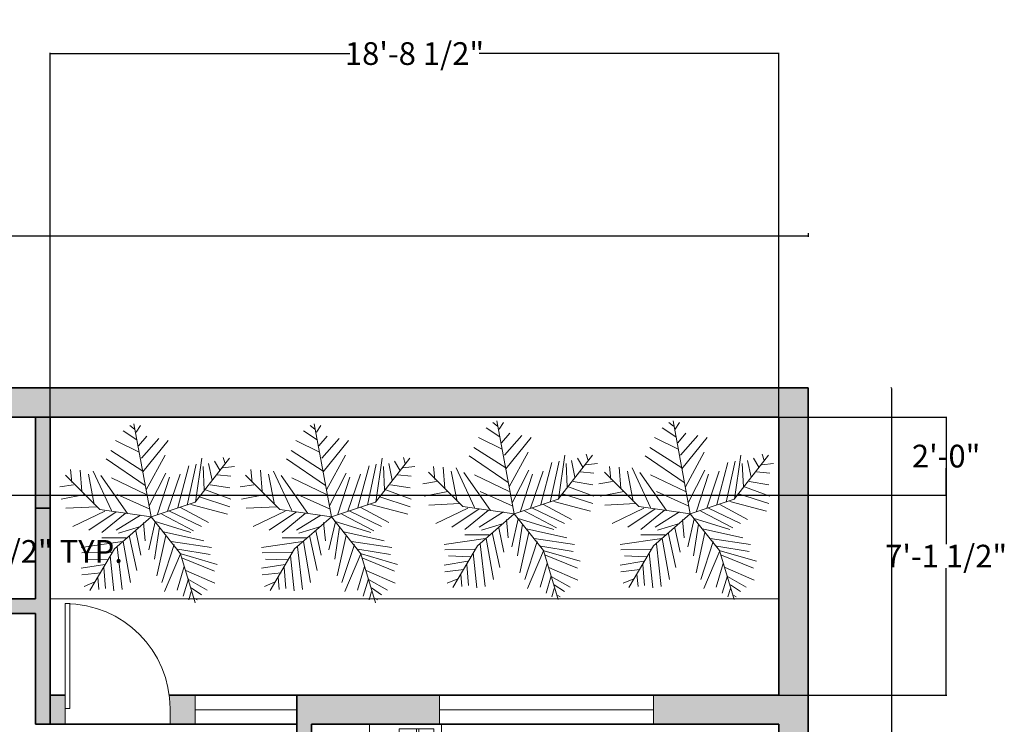
# Model space of a CAD drawing. Units: inches. Extents: x 1319 to 2030, y 219 to 1069.
# Tile 28 of 28: x 1727 to 2030, y 852 to 1069. Entities that reach past the tile are written whole.
import ezdxf

# ---------------------------------------------------------------- set-up
doc = ezdxf.new("R2010")
doc.units = ezdxf.units.IN
doc.header["$MEASUREMENT"] = 0
doc.layers.get('0').update_dxf_attribs({"color": 12})
for name, color, linetype, lineweight in [('A-ANNO-DIMS', 2, 'Continuous', 18), ('A-GLAZ', 4, 'Continuous', 18), ('A-WALL-PATT', 252, 'Continuous', 13), ('C-PROP', 7, 'Continuous', 35), ('doors', 252, 'Continuous', 18), ('furniture', 250, 'Continuous', 18), ('lawn', 82, 'Continuous', 13), ('walls', 250, 'Continuous', 35)]:
    doc.layers.add(name, color=color, linetype=linetype, lineweight=lineweight)
doc.styles.get("Standard").update_dxf_attribs({"font": 'arial.ttf'})
doc.dimstyles.get("Standard").update_dxf_attribs({"dimtxt": 7, "dimasz": 0.18, "dimexe": 0.18, "dimexo": 0.0625, "dimgap": 0.09, "dimtad": 0, "dimtih": 1, "dimtoh": 1, "dimzin": 0, "dimdsep": 46, "dimlunit": 3, "dimtxsty": 'Standard', "dimcen": 0.09, "dimadec": 0, "dimazin": 0, "dimtfac": 1, "dimtofl": 0, "dimtmove": 0, "dimatfit": 3, "dimfxl": 1, "dimtolj": 1, "dimtzin": 0, "dimarcsym": 0})

# ---------------------------------------------------------------- blocks, each defined once
blk = doc.blocks.new('*U2')
for p, q in [((0, 0), (0, -6)), ((40, 0), (40, -6))]:
    blk.add_line(p, q)
blk.add_lwpolyline([(0, 0), (0, 40), (1.75, 40), (1.75, 0)], close=True)
blk.add_arc((0, 0), 40, 0, 90)
blk = doc.blocks.new('*U27')
for p, q in [((-10.186, 53.64), (-13.084, 55.962)), ((0, 0), (-10.5, 57)), ((-9.099, 51.782), (-6.563, 55.962)), ((-8.737, 47.138), (-17.069, 52.711)), ((-7.65, 43.423), (-2.578, 49.46)), ((-7.288, 39.707), (-21.778, 46.673)), ((-5.839, 35.992), (4.667, 48.067)), ((-5.114, 27.632), (10.463, 46.673)), ((-5.114, 28.097), (-24.676, 40.636)), ((-2.941, 16.486), (8.652, 37.85)), ((44.153, 36.456), (45.239, 32.741)), ((-3.665, 19.273), (-27.574, 35.527)), ((16.259, 5.805), (23.142, 31.348)), ((22.055, 7.198), (27.489, 32.277)), ((27, 9), (48, 36)), ((27.127, 9.056), (31.112, 35.992)), ((31.836, 30.883), (32.561, 16.486)), ((35.096, 32.741), (37.27, 22.524)), ((38.719, 34.134), (41.979, 28.561)), ((43.791, 29.954), (51.036, 30.883)), ((-31.5, 4.5), (-52.5, 25.5)), ((-48.585, 21.131), (-49.309, 29.026)), ((-43.513, 28.561), (-42.427, 15.558)), ((-38.442, 26.239), (-34.819, 7.663)), ((-35.544, 28.097), (-24.314, 3.947)), ((-14.533, 2.09), (-30.834, 25.31)), ((-1.129, 6.734), (9.014, 26.704)), ((3.942, 1.625), (11.187, 24.381)), ((10.101, 3.483), (17.708, 26.239)), ((40.53, 25.775), (48.862, 24.846)), ((-47.498, 19.737), (-55.83, 18.344)), ((-24.314, 23.917), (-2.941, 13.7)), ((36.183, 19.737), (48.137, 17.88)), ((-40.615, 13.7), (-55.105, 10.913)), ((-20.691, 13.7), (-1.129, 4.876)), ((29.662, 12.307), (48.137, 6.269)), ((33.285, 16.486), (48.862, 10.913)), ((-33.37, 6.269), (-52.207, 5.34)), ((0, 0), (27, 9)), ((24.229, 7.663), (46.688, 1.625)), ((-28.299, 3.483), (-47.86, -5.805)), ((-21.416, 3.018), (-38.079, -8.128)), ((0, 0), (-31.5, 4.5)), ((-15.982, 2.09), (-30.11, -9.521)), ((0, 0), (-22.5, -19.5)), ((-6.563, 1.161), (-21.416, -8.128)), ((0, 0), (18, -22.5)), ((6.478, 1.625), (26.04, -8.592)), ((11.187, 3.483), (30.749, -5.805)), ((18.07, 5.805), (35.096, -3.483)), ((-6.563, -5.805), (-19.967, -9.985)), ((-4.752, -3.483), (-3.665, -14.629)), ((2.493, -3.019), (-1.491, -20.202)), ((1.769, -2.555), (24.229, -9.521)), ((-13.446, -11.378), (-8.737, -32.741)), ((-9.461, -8.592), (-6.201, -23.453)), ((5.029, -6.27), (2.131, -25.775)), ((9.014, -11.378), (3.58, -35.992)), ((7.565, -9.056), (32.198, -14.629)), ((-17.431, -15.094), (-42.789, -18.809)), ((-15.257, -12.772), (-30.11, -12.772)), ((-17.069, -15.094), (-12.721, -40.172)), ((14.085, -16.951), (6.478, -40.172)), ((12.274, -15.094), (36.907, -18.809)), ((-24.314, -21.596), (-42.427, -22.06)), ((-22.5, -19.5), (-37.5, -45)), ((-25.038, -23.918), (-22.865, -45.281)), ((-20.691, -18.345), (-17.793, -44.352)), ((18.07, -22.524), (8.289, -45.745)), ((16.259, -19.738), (36.183, -22.989)), ((18, -22.5), (27, -52.5)), ((18.433, -22.524), (40.53, -29.026)), ((-28.299, -29.026), (-42.789, -31.348)), ((-26.849, -26.24), (-40.253, -25.775)), ((19.157, -25.311), (38.719, -33.206)), ((-30.834, -34.135), (-42.427, -35.528)), ((-29.023, -30.884), (-27.936, -43.887)), ((20.244, -30.419), (15.897, -44.816)), ((21.331, -32.741), (39.081, -40.636)), ((-34.457, -39.708), (-40.978, -42.494)), ((-32.646, -36.921), (-31.921, -44.352)), ((22.78, -37.85), (19.519, -48.532)), ((22.78, -38.314), (34.372, -44.816)), ((24.591, -45.745), (23.142, -50.854)), ((24.591, -43.423), (30.749, -47.603)), ((26.764, -49.925), (28.213, -50.854))]:
    blk.add_line(p, q)
blk = doc.blocks.new('*D28')
at = {"layer": 'A-ANNO-DIMS', "color": 0, "lineweight": -2, "transparency": 16777216}
for p, q in [((1369.84, 1002.94), (1369.84, 1001.77)), ((1370.02, 1001.95), (1663.81, 1001.95)), ((1969.66, 1001.95), (1675.87, 1001.95)), ((1969.84, 1002.94), (1969.84, 1001.77))]:
    blk.add_line(p, q, dxfattribs=at)
at = {"layer": 'A-ANNO-DIMS', "color": 0, "transparency": 16777216}
for points in [[(1370.02, 1001.98), (1370.02, 1001.92), (1369.84, 1001.95)], [(1969.66, 1001.98), (1969.66, 1001.92), (1969.84, 1001.95)]]:
    blk.add_solid(points, dxfattribs=at)
at = {"layer": 'Defpoints', "color": 0, "transparency": 16777216}
for p in [(1369.84, 1003), (1969.84, 1003), (1969.84, 1001.95)]:
    blk.add_point(p, dxfattribs=at)
at = {"layer": 'A-ANNO-DIMS', "color": 0, "transparency": 16777216, "insert": (1669.84, 1001.95), "char_height": 7, "attachment_point": 5}
blk.add_mtext("\\A1;50'", dxfattribs=at)
blk = doc.blocks.new('*D29')
at = {"layer": 'A-ANNO-DIMS', "color": 0, "lineweight": -2, "transparency": 16777216}
for p, q in [((1995.58, 955.23), (1995.33, 955.23)), ((1995.51, 955.05), (1995.51, 628.88)), ((1995.51, 295.41), (1995.51, 621.58)), ((1995.58, 295.23), (1995.33, 295.23))]:
    blk.add_line(p, q, dxfattribs=at)
at = {"layer": 'A-ANNO-DIMS', "color": 0, "transparency": 16777216}
for points in [[(1995.48, 955.05), (1995.54, 955.05), (1995.51, 955.23)], [(1995.48, 295.41), (1995.54, 295.41), (1995.51, 295.23)]]:
    blk.add_solid(points, dxfattribs=at)
at = {"layer": 'Defpoints', "color": 0, "transparency": 16777216}
for p in [(1995.64, 955.23), (1995.51, 295.23), (1995.64, 295.23)]:
    blk.add_point(p, dxfattribs=at)
at = {"layer": 'A-ANNO-DIMS', "color": 0, "transparency": 16777216, "insert": (1995.51, 625.23), "char_height": 7, "attachment_point": 5}
blk.add_mtext("\\A1;55'", dxfattribs=at)
blk = doc.blocks.new('PLASMA-LARGE')
at = {"layer": 'furniture'}
for p, q in [((-7.26, 0), (7.26, 0)), ((-21, -2.5), (21, -2.5)), ((-21, -2.5), (-21, -3.5)), ((-21, -3.5), (21, -3.5)), ((-18.61, -1), (18.61, -1)), ((-8, -1), (-8, -0.74)), ((-8, -3.5), (-8, -4.76)), ((-7.26, -5.5), (7.26, -5.5)), ((8, -1), (8, -0.74)), ((8, -3.5), (8, -4.76)), ((21, -2.5), (21, -3.5))]:
    blk.add_line(p, q, dxfattribs=at)
for centre, radius, start, end in [((-7.26, -0.74), 0.744, 90, 180), ((7.26, -0.74), 0.744, 0, 90), ((-13.97, -11.05), 11.07, 114.76019, 129.41749), ((-7.26, -4.76), 0.744, 180, 270), ((7.26, -4.76), 0.744, 270, 0), ((13.97, -11.05), 11.07, 50.58251, 65.23981)]:
    blk.add_arc(centre, radius, start, end, dxfattribs=at)
blk = doc.blocks.new('STUDY-STATION')
h = blk.add_hatch(color=256)
h.dxf.hatch_style = 1
h.paths.add_polyline_path([(29.65, 37, 0.288578), (17.34, 37)])
h = blk.add_hatch(color=256)
h.dxf.hatch_style = 1
h.paths.add_polyline_path([(33.33, 21.74), (24.73, 21.74), (24.73, 18.77), (33.33, 18.77)])
for p, q in [((13.58, 39.93), (0, 39.93)), ((13.58, 17.73), (13.58, 39.93)), ((20.6, 38.07), (17.92, 42.38)), ((17.92, 42.38), (21.92, 38.58)), ((27.56, 41.97), (24.23, 38.82)), ((25.39, 38.48), (27.56, 41.97)), ((13.58, 37.53), (1.44, 37.53)), ((1.44, 37.53), (1.44, 26.9)), ((17.34, 37), (17.34, 25.83)), ((26.82, 37.82), (20.17, 37.82)), ((29.65, 25.83), (29.65, 37)), ((13.58, 32.99), (1.44, 32.99)), ((1.44, 32.99), (1.44, 32.21)), ((1.44, 32.21), (13.58, 32.21)), ((13.58, 26.9), (13.58, 32.99)), ((17.34, 32.49), (15.81, 32.49)), ((15.81, 32.49), (15.81, 31.73)), ((15.81, 31.73), (17.34, 31.73)), ((17.34, 32.49), (17.34, 32.49)), ((29.65, 32.49), (31.18, 32.49)), ((31.18, 31.73), (29.65, 31.73)), ((31.18, 32.49), (31.18, 31.73)), ((1.44, 26.9), (13.58, 26.9)), ((17.34, 25.83), (29.65, 25.83)), ((14.64, 17.73), (14.64, 22.88)), ((14.64, 22.88), (34.27, 22.88)), ((24.73, 17.73), (24.73, 21.74)), ((24.73, 21.74), (33.33, 21.74)), ((33.33, 21.74), (33.33, 17.73)), ((34.27, 22.88), (34.27, 17.73)), ((24.73, 18.77), (33.33, 18.77)), ((0, 17.73), (36.53, 17.73)), ((36.53, 17.73), (36.53, 0))]:
    blk.add_line(p, q)
for centre, radius, start, end in [((23.49, 27.23), 11.55, 57.806, 122.194), ((23.49, 25.83), 0.688, 180, 0)]:
    blk.add_arc(centre, radius, start, end)
at = {"xscale": -0.3577737849257557, "yscale": 0.3577737849257557, "zscale": 0.3577737849257557, "rotation": 180}
blk.add_blockref('PLASMA-LARGE', (19.61, 8.15), dxfattribs=at)
blk = doc.blocks.new('*D40')
at = {"layer": 'A-ANNO-DIMS', "color": 0, "lineweight": -2, "transparency": 16777216}
for p, q in [((1703.84, 919.51), (1708.35, 919.51)), ((1708.17, 919.33), (1708.17, 908.58)), ((1708.17, 890.41), (1708.17, 901.15)), ((1703.84, 890.23), (1708.35, 890.23))]:
    blk.add_line(p, q, dxfattribs=at)
at = {"layer": 'A-ANNO-DIMS', "color": 0, "transparency": 16777216}
for points in [[(1708.14, 919.33), (1708.2, 919.33), (1708.17, 919.51)], [(1708.14, 890.41), (1708.2, 890.41), (1708.17, 890.23)]]:
    blk.add_solid(points, dxfattribs=at)
at = {"layer": 'Defpoints', "color": 0, "transparency": 16777216}
for p in [(1703.78, 919.51), (1703.78, 890.23), (1708.17, 890.23)]:
    blk.add_point(p, dxfattribs=at)
at = {"layer": 'A-ANNO-DIMS', "color": 0, "transparency": 16777216, "insert": (1708.17, 904.87), "char_height": 7, "attachment_point": 5}
blk.add_mtext('\\A1;SHOWER 2\'-5 1/2" TYP.', dxfattribs=at)
blk = doc.blocks.new('*D67')
at = {"layer": 'A-ANNO-DIMS', "color": 0, "lineweight": -2, "transparency": 16777216}
for p, q in [((1736.34, 946.29), (1736.34, 1058.4)), ((1736.52, 1058.22), (1828.65, 1058.22)), ((1960.66, 1058.22), (1868.53, 1058.22)), ((1960.84, 946.29), (1960.84, 1058.4))]:
    blk.add_line(p, q, dxfattribs=at)
at = {"layer": 'A-ANNO-DIMS', "color": 0, "transparency": 16777216}
for points in [[(1736.52, 1058.25), (1736.52, 1058.19), (1736.34, 1058.22)], [(1960.66, 1058.25), (1960.66, 1058.19), (1960.84, 1058.22)]]:
    blk.add_solid(points, dxfattribs=at)
at = {"layer": 'Defpoints', "color": 0, "transparency": 16777216}
for p in [(1960.84, 1058.22), (1736.34, 946.23), (1960.84, 946.23)]:
    blk.add_point(p, dxfattribs=at)
at = {"layer": 'A-ANNO-DIMS', "color": 0, "transparency": 16777216, "insert": (1848.59, 1058.22), "char_height": 7, "attachment_point": 5}
blk.add_mtext('\\A1;18\'-8 1/2"', dxfattribs=at)
blk = doc.blocks.new('*D68')
at = {"layer": 'A-ANNO-DIMS', "color": 0, "lineweight": -2, "transparency": 16777216}
for p, q in [((1960.91, 946.23), (2012.57, 946.23)), ((2012.39, 946.05), (2012.39, 907.13)), ((2012.39, 860.8), (2012.39, 899.71)), ((1960.91, 860.62), (2012.57, 860.62))]:
    blk.add_line(p, q, dxfattribs=at)
at = {"layer": 'A-ANNO-DIMS', "color": 0, "transparency": 16777216}
for points in [[(2012.36, 946.05), (2012.42, 946.05), (2012.39, 946.23)], [(2012.36, 860.8), (2012.42, 860.8), (2012.39, 860.62)]]:
    blk.add_solid(points, dxfattribs=at)
at = {"layer": 'Defpoints', "color": 0, "transparency": 16777216}
for p in [(1960.84, 946.23), (1960.84, 860.62), (2012.39, 860.62)]:
    blk.add_point(p, dxfattribs=at)
at = {"layer": 'A-ANNO-DIMS', "color": 0, "transparency": 16777216, "insert": (2012.39, 903.42), "char_height": 7, "attachment_point": 5}
blk.add_mtext('\\A1;7\'-1 1/2"', dxfattribs=at)
blk = doc.blocks.new('*D71')
at = {"layer": 'A-ANNO-DIMS', "color": 0, "lineweight": -2, "transparency": 16777216}
for p, q in [((1714.83, 946.23), (2012.57, 946.23)), ((2012.39, 946.05), (2012.39, 937.89)), ((2012.39, 922.41), (2012.39, 930.56)), ((1719.33, 922.23), (2012.57, 922.23))]:
    blk.add_line(p, q, dxfattribs=at)
at = {"layer": 'A-ANNO-DIMS', "color": 0, "transparency": 16777216}
for points in [[(2012.36, 946.05), (2012.42, 946.05), (2012.39, 946.23)], [(2012.36, 922.41), (2012.42, 922.41), (2012.39, 922.23)]]:
    blk.add_solid(points, dxfattribs=at)
at = {"layer": 'Defpoints', "color": 0, "transparency": 16777216}
for p in [(1714.77, 946.23), (2012.39, 946.23), (1719.27, 922.23)]:
    blk.add_point(p, dxfattribs=at)
at = {"layer": 'A-ANNO-DIMS', "color": 0, "transparency": 16777216, "insert": (2012.39, 934.23), "char_height": 7, "attachment_point": 5}
blk.add_mtext('\\A1;2\'-0"', dxfattribs=at)

msp = doc.modelspace()

# ---------------------------------------------------------------- hatches: boundary and pattern name
at = {"layer": 'A-WALL-PATT'}
h = msp.add_hatch(color=256, dxfattribs=at)
h.dxf.hatch_style = 1
h.paths.add_polyline_path([(1378.843, 946.227), (1960.843, 946.227), (1960.843, 860.616), (1922.194, 860.616), (1922.194, 851.616), (1960.843, 851.616), (1960.843, 304.227), (1578.343, 304.227), (1578.343, 295.227), (1969.843, 295.227), (1969.843, 955.227), (1369.843, 955.227), (1369.843, 295.227), (1378.843, 295.227)])
h = msp.add_hatch(color=256, dxfattribs=at)
h.dxf.hatch_style = 1
h.paths.add_polyline_path([(1856.292, 860.616), (1812.343, 860.616), (1812.343, 851.616), (1812.343, 700.993), (1816.843, 700.993), (1816.843, 851.616), (1856.292, 851.616)])
h.paths.add_polyline_path([(1960.843, 663.616), (1812.343, 663.616), (1782.783, 663.616), (1782.783, 659.116), (1812.343, 659.116), (1960.843, 659.116)])
h.paths.add_polyline_path([(1857.424, 659.116), (1852.924, 659.116), (1852.924, 616.807), (1857.424, 616.807)])
h.paths.add_polyline_path([(1735.843, 661.727), (1731.843, 661.727), (1636.133, 661.727), (1636.133, 657.227), (1731.343, 657.227), (1731.343, 481.227), (1618.616, 481.227), (1618.616, 472.227), (1639.343, 472.227), (1639.343, 384.227), (1627.044, 384.227), (1627.044, 375.227), (1648.343, 375.227), (1648.343, 384.227), (1648.343, 472.227), (1750.706, 472.227), (1750.706, 481.227), (1735.843, 481.227), (1735.843, 657.727)])
h.paths.add_polyline_path([(1587.343, 481.227), (1578.343, 481.227), (1578.343, 375.227), (1597.622, 375.227), (1597.622, 384.227), (1587.343, 384.227)])
h.paths.add_polyline_path([(1769.593, 384.227), (1693.482, 384.227), (1693.482, 375.227), (1769.593, 375.227)])
h.paths.add_polyline_path([(1775.828, 481.227), (1765.831, 481.227), (1765.831, 472.227), (1775.828, 472.227)])
h.paths.add_polyline_path([(1824.625, 481.227), (1820.343, 481.227), (1820.343, 476.727), (1824.625, 476.727), (1824.625, 477.545)], flags=0)
h.paths.add_polyline_path([(1896.843, 481.227), (1852.26, 481.227), (1852.26, 476.727), (1892.343, 476.727), (1892.343, 384.227), (1881.742, 384.227), (1881.742, 375.227), (1913.435, 375.227), (1913.435, 384.227), (1896.843, 384.227)])
h.paths.add_polyline_path([(1960.843, 481.227), (1931.341, 481.227), (1931.341, 476.727), (1960.843, 476.727)])
h.paths.add_polyline_path([(1736.343, 918.227), (1731.843, 918.227), (1731.843, 890.227), (1582.843, 890.227), (1582.843, 781.727), (1582.843, 769.171), (1587.343, 769.171), (1587.343, 781.727), (1587.343, 885.727), (1731.843, 885.727), (1731.843, 851.616), (1736.343, 851.616), (1736.343, 890.227)])
h.paths.add_polyline_path([(1781.022, 860.616), (1773.021, 860.616, -0.0322281), (1773.289, 856.464), (1773.289, 851.616), (1781.022, 851.616)])
h.paths.add_polyline_path([(1587.343, 946.227), (1582.843, 946.227), (1582.843, 926.136), (1587.343, 926.136)])
h.paths.add_polyline_path([(1647.843, 946.227), (1643.343, 946.227), (1643.343, 926.136), (1647.843, 926.136)])
h.paths.add_polyline_path([(1543.343, 786.227), (1429.843, 786.227), (1429.843, 757.555), (1434.343, 757.555), (1438.843, 757.555), (1438.843, 781.727), (1543.343, 781.727)])
h.paths.add_polyline_path([(1543.343, 781.727), (1538.843, 781.727), (1538.843, 709.727), (1534.597, 709.727), (1534.597, 705.227), (1543.343, 705.227), (1543.343, 709.727)])
h.paths.add_polyline_path([(1499.955, 709.727), (1438.843, 709.727), (1438.843, 734.463), (1429.843, 734.463), (1429.843, 552.227), (1470.241, 552.227), (1470.241, 561.227), (1438.843, 561.227), (1438.843, 705.227), (1499.955, 705.227)])
h.paths.add_polyline_path([(1587.343, 709.727), (1582.843, 709.727), (1582.843, 561.227), (1543.433, 561.227), (1543.433, 552.227), (1587.343, 552.227)])
h.paths.add_polyline_path([(1546.835, 709.727), (1543.343, 709.727), (1543.343, 705.227), (1546.835, 705.227)])
h.paths.add_polyline_path([(1582.843, 709.727), (1579.15, 709.727), (1579.15, 705.227), (1582.843, 705.227)], flags=17)
h.paths.add_polyline_path([(1548.368, 786.227), (1543.343, 786.227), (1543.343, 781.727), (1548.368, 781.727)])
h.paths.add_polyline_path([(1582.843, 786.227), (1580.683, 786.227), (1580.683, 781.727), (1582.843, 781.727)])
h.paths.add_polyline_path([(1587.343, 892.402), (1582.843, 892.402), (1582.843, 890.227), (1587.343, 890.227)], flags=17)
h.paths.add_polyline_path([(1647.843, 892.402), (1643.343, 892.402), (1643.343, 890.227), (1647.843, 890.227)], flags=17)
h.paths.add_polyline_path([(1740.974, 856.464), (1740.974, 860.616), (1736.343, 860.616), (1736.343, 851.616), (1740.974, 851.616)])
h.paths.add_polyline_path([(1853.989, 384.227), (1820.343, 384.227), (1820.343, 402.924), (1815.843, 402.924), (1815.843, 375.227), (1853.989, 375.227)])
h.paths.add_polyline_path([(1892.343, 436.227), (1820.343, 436.227), (1820.343, 481.227), (1815.843, 481.227), (1815.843, 431.727), (1892.343, 431.727)])
h.paths.add_polyline_path([(1849.175, 481.227), (1824.625, 481.227), (1824.625, 477.545), (1825.699, 477.545), (1825.699, 453.018, 0.4014527), (1849.175, 477.545)], flags=0)
h.paths.add_polyline_path([(1960.843, 384.227), (1941.188, 384.227), (1941.188, 375.227), (1960.843, 375.227)])
h.paths.add_polyline_path([(1902.267, 481.227), (1896.843, 481.227), (1896.843, 476.727), (1902.267, 476.727), (1902.267, 477.44)], flags=0)
h = msp.add_hatch(color=256, dxfattribs=at)
h.dxf.hatch_style = 1
h.paths.add_polyline_path([(1736.343, 946.227), (1731.843, 946.227), (1731.843, 918.227), (1736.343, 918.227)])

# ---------------------------------------------------------------- linework, layer by layer
at = {"layer": 'A-GLAZ'}
for p, q in [((1781.022, 851.616), (1781.022, 860.616)), ((1781.022, 860.616), (1812.343, 860.616)), ((1812.343, 860.616), (1812.343, 851.616)), ((1812.343, 860.616), (1812.343, 851.616)), ((1856.292, 860.616), (1856.292, 851.616)), ((1922.194, 860.616), (1856.292, 860.616)), ((1856.292, 860.616), (1856.292, 856.116)), ((1922.194, 851.616), (1922.194, 860.616)), ((1812.343, 856.116), (1781.022, 856.116)), ((1812.343, 851.616), (1812.343, 856.116)), ((1856.292, 856.116), (1922.194, 856.116)), ((1812.343, 851.616), (1781.022, 851.616)), ((1856.292, 851.616), (1922.194, 851.616))]:
    msp.add_line(p, q, dxfattribs=at)
at = {"layer": 'C-PROP'}
for p, q in [((1369.843, 955.227), (1969.843, 955.227)), ((1969.843, 955.227), (1969.843, 295.227))]:
    msp.add_line(p, q, dxfattribs=at)
at = {"layer": 'lawn'}
msp.add_line((1736.343, 890.227), (1960.843, 890.227), dxfattribs=at)
at = {"layer": 'walls'}
for p, q in [((1378.843, 946.227), (1960.843, 946.227)), ((1731.843, 890.227), (1731.843, 946.227)), ((1736.343, 890.227), (1736.343, 946.227)), ((1960.843, 946.227), (1960.843, 860.616)), ((1731.843, 918.227), (1736.343, 918.227)), ((1582.843, 890.227), (1731.843, 890.227)), ((1736.343, 851.616), (1736.343, 890.227)), ((1587.343, 885.727), (1731.843, 885.727)), ((1731.843, 885.727), (1731.843, 851.616)), ((1731.843, 851.616), (1731.843, 860.616)), ((1736.343, 860.616), (1740.974, 860.616)), ((1773.021, 860.616), (1960.843, 860.616)), ((1812.343, 860.616), (1812.343, 663.616)), ((1731.843, 851.616), (1736.343, 851.616)), ((1736.343, 851.616), (1812.343, 851.616)), ((1816.843, 851.616), (1816.843, 698.031)), ((1816.843, 851.616), (1960.843, 851.616)), ((1960.843, 851.616), (1960.843, 304.227))]:
    msp.add_line(p, q, dxfattribs=at)

# ---------------------------------------------------------------- block references
at = {"layer": 'doors', "xscale": 0.8078659498341503, "yscale": 0.8078659498341503, "zscale": 0.8078659498341503}
msp.add_blockref('*U2', (1740.974, 856.464), dxfattribs=at)
at = {"layer": 'furniture', "rotation": 269.9999999999988}
msp.add_blockref('STUDY-STATION', (1816.976, 851.616), dxfattribs=at)
at = {"layer": 'lawn', "xscale": 0.5032398725192154, "yscale": 0.5032398725192154, "zscale": 0.5032398725192154}
for p in [(1767.443, 915.498), (1822.99, 915.498), (1879.284, 916.433), (1933.527, 916.433)]:
    msp.add_blockref('*U27', p, dxfattribs=at)

# ---------------------------------------------------------------- dimensions: what is measured, and where the dimension line sits
at = {"layer": 'A-ANNO-DIMS'}
for base, p1, p2, override, picture, middle in [((1960.843, 1058.218), (1736.343, 946.227), (1960.843, 946.227), {"dimdec": 1, "dimlfac": 1, "dimrnd": 0, "dimzin": 1, "dimdsep": 46, "dimlunit": 4, "dimfrac": 2}, '*D67', (1848.593, 1058.218)), ((1969.843, 1001.954), (1369.843, 1003), (1969.843, 1003), {"dimclrd": 0, "dimclre": 0, "dimclrt": 0}, '*D28', (1669.843, 1001.954))]:
    dim = msp.add_linear_dim(base=base, p1=p1, p2=p2, dimstyle='Standard', override=override, dxfattribs=at)
    dim.commit()
    dim.dimension.update_dxf_attribs({"geometry": picture, "text_midpoint": middle})
for base, p1, p2, override, picture, middle in [((1995.506, 295.227), (1995.643, 955.227), (1995.643, 295.227), {"dimclrd": 0, "dimclre": 0, "dimclrt": 0}, '*D29', (1995.506, 625.227)), ((2012.394, 946.227), (1719.265, 922.227), (1714.765, 946.227), {"dimdec": 1, "dimlfac": 1, "dimrnd": 0, "dimzin": 1, "dimdsep": 46, "dimlunit": 4, "dimfrac": 2}, '*D71', (2012.394, 934.227)), ((2012.394, 860.616), (1960.843, 946.227), (1960.843, 860.616), {"dimdec": 1, "dimlfac": 1, "dimrnd": 0, "dimzin": 1, "dimdsep": 46, "dimlunit": 4, "dimfrac": 2}, '*D68', (2012.394, 903.422))]:
    dim = msp.add_linear_dim(base=base, p1=p1, p2=p2, angle=90, dimstyle='Standard', override=override, dxfattribs=at)
    dim.commit()
    dim.dimension.update_dxf_attribs({"geometry": picture, "text_midpoint": middle})
dim = msp.add_linear_dim(base=(1708.17, 890.227), p1=(1703.778, 919.506), p2=(1703.778, 890.227), angle=270, text='SHOWER <> TYP.', dimstyle='Standard', override={"dimdec": 1, "dimlfac": 1, "dimrnd": 0, "dimzin": 1, "dimdsep": 46, "dimlunit": 4, "dimfrac": 2}, dxfattribs=at)
dim.commit()
dim.dimension.update_dxf_attribs({"geometry": '*D40', "text_midpoint": (1708.17, 904.867)})

doc.saveas('drawing.dxf')
